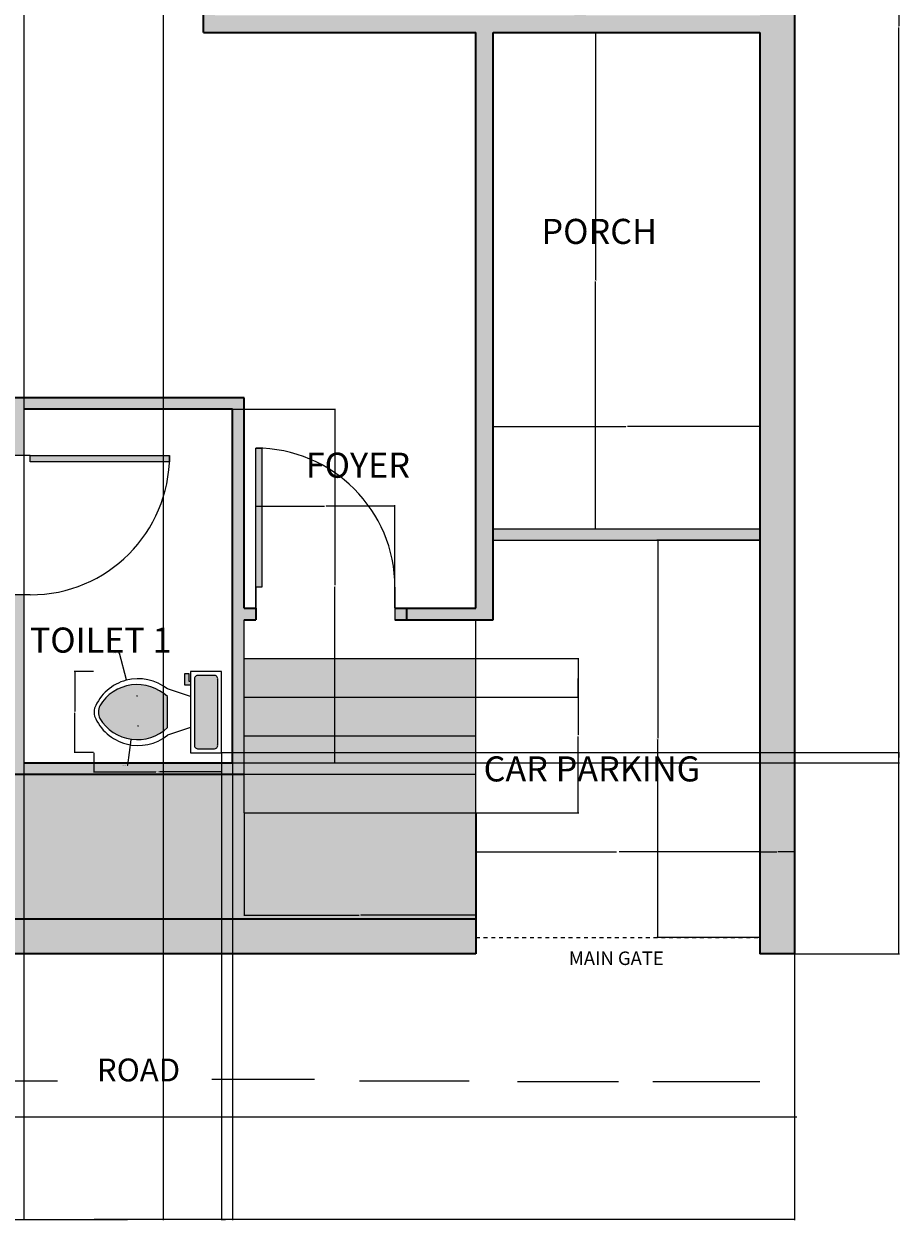
# Model space of a CAD drawing. Units: inches. Extents: x 1034 to 1730, y 674 to 1249.
# Tile 2 of 4: x 1503 to 1730, y 674 to 983. Entities that reach past the tile are written whole.
import ezdxf

# ---------------------------------------------------------------- set-up
doc = ezdxf.new("R2010")
doc.units = ezdxf.units.IN
doc.linetypes.add('JIS_02_1.0', pattern=[2, 1, -1])
for name, color, linetype, lineweight in [('A-ANNO-DIMS', 2, 'Continuous', 18), ('A-ANNO-TEXT', 7, 'Continuous', 18), ('A-AREA-IDEN', 7, 'Continuous', 18), ('A-DOOR', 4, 'Continuous', 25), ('A-FLOR', 7, 'Continuous', 25), ('A-FLOR-FIXT', 9, 'Continuous', 18), ('A-FLOR-FIXT-PATT', 7, 'Continuous', 13), ('A-FLOR-PATT', 8, 'Continuous', 13), ('A-FLOR-STRS', 7, 'Continuous', 25), ('A-FURN-PATT', 7, 'Continuous', 13), ('A-WALL', 7, 'Continuous', 35), ('A-WALL-PATT', 8, 'Continuous', 13), ('C-ROAD', 7, 'Continuous', 18), ('C-SITE-GATE', 4, 'JIS_02_1.0', 25)]:
    doc.layers.add(name, color=color, linetype=linetype, lineweight=lineweight)
for name, color, linetype, lineweight, true_color in [('A-DOOR-PATT', 17, 'Continuous', 13, 0x7b4636), ('A-FLOR-STRS-PATT', 253, 'Continuous', 13, 0xb3beaa), ('C-SITE-PATT', 18, 'Continuous', 13, 0x000000)]:
    doc.layers.add(name, color=color, linetype=linetype, lineweight=lineweight, true_color=true_color)
doc.styles.get("Standard").update_dxf_attribs({"font": 'arial.ttf'})
doc.dimstyles.get("Standard").update_dxf_attribs({"dimtxt": 0.18, "dimasz": 0.18, "dimexe": 0.18, "dimexo": 0.0625, "dimgap": 0.09, "dimtad": 0, "dimtih": 1, "dimtoh": 1, "dimdec": 4, "dimzin": 0, "dimdsep": 46, "dimtxsty": 'Standard', "dimcen": 0.09, "dimadec": 0, "dimazin": 0, "dimtfac": 1, "dimtdec": 4, "dimtofl": 0, "dimtmove": 0, "dimatfit": 3, "dimfxl": 1, "dimtolj": 1, "dimtzin": 0, "dimarcsym": 0})

# ---------------------------------------------------------------- blocks, each defined once
blk = doc.blocks.new('*U3')
for p, q in [((0, 0), (0, -6)), ((40, 0), (40, -6))]:
    blk.add_line(p, q)
blk.add_lwpolyline([(0, 0), (0, 40), (1.75, 40), (1.75, 0)], close=True)
blk.add_arc((0, 0), 40, 0, 90)
blk = doc.blocks.new('Toilet - top')
for p, q in [((9.5, -6), (9.5, -2)), ((-10, -8.5), (-8, -8.5)), ((-10, -9.5), (-10, -8.5)), ((-8, -8.5), (-8, -8)), ((-7, -8), (-7, -9.5)), ((-4, -8), (-6, -14)), ((4, -8), (6, -14)), ((-7, -9.5), (-10, -9.5)), ((4, -14), (-4, -14))]:
    blk.add_line(p, q)
blk.add_lwpolyline([(10.5, -8), (10.5, 0), (-10.5, 0), (-10.5, -8)], close=True)
for points in [[(-9.5, -2), (-9.5, -6)], [(8.5, -1), (-8.5, -1)], [(-8.5, -7), (8.5, -7)]]:
    blk.add_lwpolyline(points)
for centre, radius, start, end in [((-8.62, -1.88), 0.884, 81.8699, 188.1301), ((8.62, -1.88), 0.884, 351.8699, 98.1301), ((-8.62, -6.12), 0.884, 171.8699, 278.1301), ((8.62, -6.12), 0.884, 261.8699, 8.1301), ((3.52, -21.58), 12.17, 141.4691, 247.9714), ((4.2, -21.82), 11.33, 136.3677, 238.9468), ((-3.52, -21.58), 12.17, 292.0284, 38.5307), ((-4.2, -21.82), 11.33, 301.053, 43.6321), ((0, -27.88), 4, 245.7318, 294.2682), ((0, -29), 4, 254.8605, 285.1395)]:
    blk.add_arc(centre, radius, start, end)
blk = doc.blocks.new('*D10')
at = {"layer": 'A-ANNO-DIMS', "color": 0, "lineweight": -2, "transparency": 16777216}
for p, q in [((1521.14, 794.46), (1521.14, 789.39)), ((1554.18, 794.46), (1554.18, 789.39)), ((1521.32, 789.57), (1537.19, 789.57)), ((1554, 789.57), (1538.13, 789.57))]:
    blk.add_line(p, q, dxfattribs=at)
at = {"layer": 'A-ANNO-DIMS', "color": 0, "transparency": 16777216}
for points in [[(1521.32, 789.6), (1521.32, 789.54), (1521.14, 789.57)], [(1554, 789.6), (1554, 789.54), (1554.18, 789.57)]]:
    blk.add_solid(points, dxfattribs=at)
at = {"layer": 'Defpoints', "color": 0, "transparency": 16777216}
for p in [(1521.14, 794.53), (1554.18, 794.53), (1554.18, 789.57)]:
    blk.add_point(p, dxfattribs=at)
at = {"layer": 'A-ANNO-DIMS', "color": 0, "transparency": 16777216, "insert": (1537.66, 789.57), "char_height": 0.18, "attachment_point": 5}
blk.add_mtext('\\A1;WC 33', dxfattribs=at)
blk = doc.blocks.new('*D11')
at = {"layer": 'A-ANNO-DIMS', "color": 0, "lineweight": -2, "transparency": 16777216}
for p, q in [((1521.07, 815.53), (1516, 815.53)), ((1516.18, 815.35), (1516.18, 805.21)), ((1516.18, 794.71), (1516.18, 804.85)), ((1521.07, 794.53), (1516, 794.53))]:
    blk.add_line(p, q, dxfattribs=at)
at = {"layer": 'A-ANNO-DIMS', "color": 0, "transparency": 16777216}
for points in [[(1516.15, 815.35), (1516.21, 815.35), (1516.18, 815.53)], [(1516.15, 794.71), (1516.21, 794.71), (1516.18, 794.53)]]:
    blk.add_solid(points, dxfattribs=at)
at = {"layer": 'Defpoints', "color": 0, "transparency": 16777216}
for p in [(1521.14, 815.53), (1516.18, 794.53), (1521.14, 794.53)]:
    blk.add_point(p, dxfattribs=at)
at = {"layer": 'A-ANNO-DIMS', "color": 0, "transparency": 16777216, "insert": (1516.18, 805.03), "char_height": 0.18, "attachment_point": 5}
blk.add_mtext('\\A1;21', dxfattribs=at)
blk = doc.blocks.new('*D14')
at = {"layer": 'A-ANNO-DIMS', "color": 0, "lineweight": -2, "transparency": 16777216}
for p, q in [((1342.53, 742.36), (1342.53, 673.53)), ((1702.53, 742.36), (1702.53, 673.53)), ((1342.71, 673.71), (1522.24, 673.71)), ((1702.35, 673.71), (1522.82, 673.71))]:
    blk.add_line(p, q, dxfattribs=at)
at = {"layer": 'A-ANNO-DIMS', "color": 0, "transparency": 16777216}
for points in [[(1342.71, 673.74), (1342.71, 673.68), (1342.53, 673.71)], [(1702.35, 673.74), (1702.35, 673.68), (1702.53, 673.71)]]:
    blk.add_solid(points, dxfattribs=at)
at = {"layer": 'Defpoints', "color": 0, "transparency": 16777216}
for p in [(1342.53, 742.43), (1702.53, 742.43), (1702.53, 673.71)]:
    blk.add_point(p, dxfattribs=at)
at = {"layer": 'A-ANNO-DIMS', "color": 0, "transparency": 16777216, "insert": (1522.53, 673.71), "char_height": 0.18, "attachment_point": 5}
blk.add_mtext('\\A1;360', dxfattribs=at)
blk = doc.blocks.new('*D15')
at = {"layer": 'A-ANNO-DIMS', "color": 0, "lineweight": -2, "transparency": 16777216}
for p, q in [((1702.59, 1222.43), (1729.69, 1222.43)), ((1729.51, 1222.25), (1729.51, 982.61)), ((1729.51, 742.61), (1729.51, 982.24)), ((1702.59, 742.43), (1729.69, 742.43))]:
    blk.add_line(p, q, dxfattribs=at)
at = {"layer": 'A-ANNO-DIMS', "color": 0, "transparency": 16777216}
for points in [[(1729.48, 1222.25), (1729.54, 1222.25), (1729.51, 1222.43)], [(1729.48, 742.61), (1729.54, 742.61), (1729.51, 742.43)]]:
    blk.add_solid(points, dxfattribs=at)
at = {"layer": 'Defpoints', "color": 0, "transparency": 16777216}
for p in [(1702.53, 1222.43), (1729.51, 1222.43), (1702.53, 742.43)]:
    blk.add_point(p, dxfattribs=at)
at = {"layer": 'A-ANNO-DIMS', "color": 0, "transparency": 16777216, "insert": (1729.51, 982.43), "char_height": 0.18, "attachment_point": 5}
blk.add_mtext('\\A1;480', dxfattribs=at)
blk = doc.blocks.new('*D24')
at = {"layer": 'A-ANNO-DIMS', "color": 0, "lineweight": -2, "transparency": 16777216}
for p, q in [((1624.53, 852.56), (1624.53, 879.13)), ((1624.71, 878.95), (1658.81, 878.95)), ((1693.35, 878.95), (1659.25, 878.95)), ((1693.53, 852.56), (1693.53, 879.13))]:
    blk.add_line(p, q, dxfattribs=at)
at = {"layer": 'A-ANNO-DIMS', "color": 0, "transparency": 16777216}
for points in [[(1624.71, 878.98), (1624.71, 878.92), (1624.53, 878.95)], [(1693.35, 878.98), (1693.35, 878.92), (1693.53, 878.95)]]:
    blk.add_solid(points, dxfattribs=at)
at = {"layer": 'Defpoints', "color": 0, "transparency": 16777216}
for p in [(1693.53, 878.95), (1624.53, 852.5), (1693.53, 852.5)]:
    blk.add_point(p, dxfattribs=at)
at = {"layer": 'A-ANNO-DIMS', "color": 0, "transparency": 16777216, "insert": (1659.03, 878.95), "char_height": 0.18, "attachment_point": 5}
blk.add_mtext('\\A1;69', dxfattribs=at)
blk = doc.blocks.new('*D25')
at = {"layer": 'A-ANNO-DIMS', "color": 0, "lineweight": -2, "transparency": 16777216}
for p, q in [((1624.59, 980.93), (1651.16, 980.93)), ((1650.98, 980.75), (1650.98, 916.9)), ((1650.98, 852.68), (1650.98, 916.53)), ((1624.59, 852.5), (1651.16, 852.5))]:
    blk.add_line(p, q, dxfattribs=at)
at = {"layer": 'A-ANNO-DIMS', "color": 0, "transparency": 16777216}
for points in [[(1650.95, 980.75), (1651.01, 980.75), (1650.98, 980.93)], [(1650.95, 852.68), (1651.01, 852.68), (1650.98, 852.5)]]:
    blk.add_solid(points, dxfattribs=at)
at = {"layer": 'Defpoints', "color": 0, "transparency": 16777216}
for p in [(1624.53, 980.93), (1624.53, 852.5), (1650.98, 852.5)]:
    blk.add_point(p, dxfattribs=at)
at = {"layer": 'A-ANNO-DIMS', "color": 0, "transparency": 16777216, "insert": (1650.98, 916.71), "char_height": 0.18, "attachment_point": 5}
blk.add_mtext('\\A1;128.42', dxfattribs=at)
blk = doc.blocks.new('*D28')
at = {"layer": 'A-ANNO-DIMS', "color": 0, "lineweight": -2, "transparency": 16777216}
for p, q in [((1503.03, 1153.36), (1503.03, 673.53)), ((1539.03, 1153.36), (1539.03, 673.53)), ((1503.21, 673.71), (1520.81, 673.71)), ((1538.85, 673.71), (1521.25, 673.71))]:
    blk.add_line(p, q, dxfattribs=at)
at = {"layer": 'A-ANNO-DIMS', "color": 0, "transparency": 16777216}
for points in [[(1503.21, 673.74), (1503.21, 673.68), (1503.03, 673.71)], [(1538.85, 673.74), (1538.85, 673.68), (1539.03, 673.71)]]:
    blk.add_solid(points, dxfattribs=at)
at = {"layer": 'Defpoints', "color": 0, "transparency": 16777216}
for p in [(1503.03, 1153.43), (1539.03, 1153.43), (1539.03, 673.71)]:
    blk.add_point(p, dxfattribs=at)
at = {"layer": 'A-ANNO-DIMS', "color": 0, "transparency": 16777216, "insert": (1521.03, 673.71), "char_height": 0.18, "attachment_point": 5}
blk.add_mtext('\\A1;36', dxfattribs=at)
blk = doc.blocks.new('*D29')
at = {"layer": 'A-ANNO-DIMS', "color": 0, "lineweight": -2, "transparency": 16777216}
for p, q in [((1503.03, 791.86), (1503.03, 673.53)), ((1557.03, 791.86), (1557.03, 673.53)), ((1503.21, 673.71), (1529.81, 673.71)), ((1556.85, 673.71), (1530.25, 673.71))]:
    blk.add_line(p, q, dxfattribs=at)
at = {"layer": 'A-ANNO-DIMS', "color": 0, "transparency": 16777216}
for points in [[(1503.21, 673.74), (1503.21, 673.68), (1503.03, 673.71)], [(1556.85, 673.74), (1556.85, 673.68), (1557.03, 673.71)]]:
    blk.add_solid(points, dxfattribs=at)
at = {"layer": 'Defpoints', "color": 0, "transparency": 16777216}
for p in [(1503.03, 791.93), (1557.03, 791.93), (1557.03, 673.71)]:
    blk.add_point(p, dxfattribs=at)
at = {"layer": 'A-ANNO-DIMS', "color": 0, "transparency": 16777216, "insert": (1530.03, 673.71), "char_height": 0.18, "attachment_point": 5}
blk.add_mtext('\\A1;54', dxfattribs=at)
blk = doc.blocks.new('*D30')
at = {"layer": 'A-ANNO-DIMS', "color": 0, "lineweight": -2, "transparency": 16777216}
for p, q in [((1557.09, 883.43), (1583.66, 883.43)), ((1583.48, 883.25), (1583.48, 837.86)), ((1583.48, 792.11), (1583.48, 837.49)), ((1557.09, 791.93), (1583.66, 791.93))]:
    blk.add_line(p, q, dxfattribs=at)
at = {"layer": 'A-ANNO-DIMS', "color": 0, "transparency": 16777216}
for points in [[(1583.45, 883.25), (1583.51, 883.25), (1583.48, 883.43)], [(1583.45, 792.11), (1583.51, 792.11), (1583.48, 791.93)]]:
    blk.add_solid(points, dxfattribs=at)
at = {"layer": 'Defpoints', "color": 0, "transparency": 16777216}
for p in [(1557.03, 883.43), (1557.03, 791.93), (1583.48, 791.93)]:
    blk.add_point(p, dxfattribs=at)
at = {"layer": 'A-ANNO-DIMS', "color": 0, "transparency": 16777216, "insert": (1583.48, 837.68), "char_height": 0.18, "attachment_point": 5}
blk.add_mtext('\\A1;91.5', dxfattribs=at)
blk = doc.blocks.new('*D39')
at = {"layer": 'A-ANNO-DIMS', "color": 0, "lineweight": -2, "transparency": 16777216}
for p, q in [((1620.03, 742.49), (1620.03, 769.06)), ((1620.21, 768.88), (1656.46, 768.88)), ((1693.35, 768.88), (1657.1, 768.88)), ((1693.53, 742.49), (1693.53, 769.06))]:
    blk.add_line(p, q, dxfattribs=at)
at = {"layer": 'A-ANNO-DIMS', "color": 0, "transparency": 16777216}
for points in [[(1620.21, 768.91), (1620.21, 768.85), (1620.03, 768.88)], [(1693.35, 768.91), (1693.35, 768.85), (1693.53, 768.88)]]:
    blk.add_solid(points, dxfattribs=at)
at = {"layer": 'Defpoints', "color": 0, "transparency": 16777216}
for p in [(1693.53, 768.88), (1620.03, 742.43), (1693.53, 742.43)]:
    blk.add_point(p, dxfattribs=at)
at = {"layer": 'A-ANNO-DIMS', "color": 0, "transparency": 16777216, "insert": (1656.78, 768.88), "char_height": 0.18, "attachment_point": 5}
blk.add_mtext('\\A1;73.5', dxfattribs=at)
blk = doc.blocks.new('*D40')
at = {"layer": 'A-ANNO-DIMS', "color": 0, "lineweight": -2, "transparency": 16777216}
for p, q in [((1560.03, 778.86), (1560.03, 752.3)), ((1620.03, 778.86), (1620.03, 752.3)), ((1560.21, 752.48), (1589.81, 752.48)), ((1619.85, 752.48), (1590.25, 752.48))]:
    blk.add_line(p, q, dxfattribs=at)
at = {"layer": 'A-ANNO-DIMS', "color": 0, "transparency": 16777216}
for points in [[(1560.21, 752.51), (1560.21, 752.45), (1560.03, 752.48)], [(1619.85, 752.51), (1619.85, 752.45), (1620.03, 752.48)]]:
    blk.add_solid(points, dxfattribs=at)
at = {"layer": 'Defpoints', "color": 0, "transparency": 16777216}
for p in [(1560.03, 778.93), (1620.03, 778.93), (1560.03, 752.48)]:
    blk.add_point(p, dxfattribs=at)
at = {"layer": 'A-ANNO-DIMS', "color": 0, "transparency": 16777216, "insert": (1590.03, 752.48), "char_height": 0.18, "attachment_point": 5}
blk.add_mtext('\\A1;60', dxfattribs=at)
blk = doc.blocks.new('*D41')
at = {"layer": 'A-ANNO-DIMS', "color": 0, "lineweight": -2, "transparency": 16777216}
for p, q in [((1693.53, 742.49), (1693.53, 769.06)), ((1693.71, 768.88), (1697.88, 768.88)), ((1702.35, 768.88), (1698.18, 768.88)), ((1702.53, 742.49), (1702.53, 769.06))]:
    blk.add_line(p, q, dxfattribs=at)
at = {"layer": 'A-ANNO-DIMS', "color": 0, "transparency": 16777216}
for points in [[(1693.71, 768.91), (1693.71, 768.85), (1693.53, 768.88)], [(1702.35, 768.91), (1702.35, 768.85), (1702.53, 768.88)]]:
    blk.add_solid(points, dxfattribs=at)
at = {"layer": 'Defpoints', "color": 0, "transparency": 16777216}
for p in [(1702.53, 768.88), (1693.53, 742.43), (1702.53, 742.43)]:
    blk.add_point(p, dxfattribs=at)
at = {"layer": 'A-ANNO-DIMS', "color": 0, "transparency": 16777216, "insert": (1698.03, 768.88), "char_height": 0.18, "attachment_point": 5}
blk.add_mtext('\\A1;9', dxfattribs=at)
blk = doc.blocks.new('*D44')
at = {"layer": 'A-ANNO-DIMS', "color": 0, "lineweight": -2, "transparency": 16777216}
for p, q in [((1620.09, 818.93), (1646.66, 818.93)), ((1646.48, 818.75), (1646.48, 799.11)), ((1646.48, 779.11), (1646.48, 798.74)), ((1620.09, 778.93), (1646.66, 778.93))]:
    blk.add_line(p, q, dxfattribs=at)
at = {"layer": 'A-ANNO-DIMS', "color": 0, "transparency": 16777216}
for points in [[(1646.45, 818.75), (1646.51, 818.75), (1646.48, 818.93)], [(1646.45, 779.11), (1646.51, 779.11), (1646.48, 778.93)]]:
    blk.add_solid(points, dxfattribs=at)
at = {"layer": 'Defpoints', "color": 0, "transparency": 16777216}
for p in [(1620.03, 818.93), (1620.03, 778.93), (1646.48, 778.93)]:
    blk.add_point(p, dxfattribs=at)
at = {"layer": 'A-ANNO-DIMS', "color": 0, "transparency": 16777216, "insert": (1646.48, 798.93), "char_height": 0.18, "attachment_point": 5}
blk.add_mtext('\\A1;40', dxfattribs=at)
blk = doc.blocks.new('*D47')
at = {"layer": 'A-ANNO-DIMS', "color": 0, "lineweight": -2, "transparency": 16777216}
for p, q in [((1563.03, 831.99), (1563.03, 858.56)), ((1563.21, 858.38), (1580.81, 858.38)), ((1598.85, 858.38), (1581.25, 858.38)), ((1599.03, 831.99), (1599.03, 858.56))]:
    blk.add_line(p, q, dxfattribs=at)
at = {"layer": 'A-ANNO-DIMS', "color": 0, "transparency": 16777216}
for points in [[(1563.21, 858.41), (1563.21, 858.35), (1563.03, 858.38)], [(1598.85, 858.41), (1598.85, 858.35), (1599.03, 858.38)]]:
    blk.add_solid(points, dxfattribs=at)
at = {"layer": 'Defpoints', "color": 0, "transparency": 16777216}
for p in [(1599.03, 858.38), (1563.03, 831.93), (1599.03, 831.93)]:
    blk.add_point(p, dxfattribs=at)
at = {"layer": 'A-ANNO-DIMS', "color": 0, "transparency": 16777216, "insert": (1581.03, 858.38), "char_height": 0.18, "attachment_point": 5}
blk.add_mtext('\\A1;36', dxfattribs=at)
blk = doc.blocks.new('*D48')
at = {"layer": 'A-ANNO-DIMS', "color": 0, "lineweight": -2, "transparency": 16777216}
for p, q in [((1620.09, 818.93), (1646.66, 818.93)), ((1646.48, 818.75), (1646.48, 814.11)), ((1646.48, 809.11), (1646.48, 813.74)), ((1620.09, 808.93), (1646.66, 808.93))]:
    blk.add_line(p, q, dxfattribs=at)
at = {"layer": 'A-ANNO-DIMS', "color": 0, "transparency": 16777216}
for points in [[(1646.45, 818.75), (1646.51, 818.75), (1646.48, 818.93)], [(1646.45, 809.11), (1646.51, 809.11), (1646.48, 808.93)]]:
    blk.add_solid(points, dxfattribs=at)
at = {"layer": 'Defpoints', "color": 0, "transparency": 16777216}
for p in [(1620.03, 818.93), (1620.03, 808.93), (1646.48, 808.93)]:
    blk.add_point(p, dxfattribs=at)
at = {"layer": 'A-ANNO-DIMS', "color": 0, "transparency": 16777216, "insert": (1646.48, 813.93), "char_height": 0.18, "attachment_point": 5}
blk.add_mtext('\\A1;10', dxfattribs=at)
blk = doc.blocks.new('*D49')
at = {"layer": 'A-ANNO-DIMS', "color": 0, "lineweight": -2, "transparency": 16777216}
for p, q in [((1554.18, 794.46), (1554.18, 673.53)), ((1557.03, 791.86), (1557.03, 673.53)), ((1554.36, 673.71), (1555.21, 673.71)), ((1556.85, 673.71), (1556, 673.71))]:
    blk.add_line(p, q, dxfattribs=at)
at = {"layer": 'A-ANNO-DIMS', "color": 0, "transparency": 16777216}
for points in [[(1554.36, 673.74), (1554.36, 673.68), (1554.18, 673.71)], [(1556.85, 673.74), (1556.85, 673.68), (1557.03, 673.71)]]:
    blk.add_solid(points, dxfattribs=at)
at = {"layer": 'Defpoints', "color": 0, "transparency": 16777216}
for p in [(1554.18, 794.53), (1557.03, 791.93), (1557.03, 673.71)]:
    blk.add_point(p, dxfattribs=at)
at = {"layer": 'A-ANNO-DIMS', "color": 0, "transparency": 16777216, "insert": (1555.61, 673.71), "char_height": 0.18, "attachment_point": 5}
blk.add_mtext('\\A1;2.847', dxfattribs=at)
blk = doc.blocks.new('*D50')
at = {"layer": 'A-ANNO-DIMS', "color": 0, "lineweight": -2, "transparency": 16777216}
for p, q in [((1554.24, 794.53), (1729.69, 794.53)), ((1729.51, 794.35), (1729.51, 793.41)), ((1729.51, 792.11), (1729.51, 793.04)), ((1557.09, 791.93), (1729.69, 791.93))]:
    blk.add_line(p, q, dxfattribs=at)
at = {"layer": 'A-ANNO-DIMS', "color": 0, "transparency": 16777216}
for points in [[(1729.48, 794.35), (1729.54, 794.35), (1729.51, 794.53)], [(1729.48, 792.11), (1729.54, 792.11), (1729.51, 791.93)]]:
    blk.add_solid(points, dxfattribs=at)
at = {"layer": 'Defpoints', "color": 0, "transparency": 16777216}
for p in [(1554.18, 794.53), (1557.03, 791.93), (1729.51, 791.93)]:
    blk.add_point(p, dxfattribs=at)
at = {"layer": 'A-ANNO-DIMS', "color": 0, "transparency": 16777216, "insert": (1729.51, 793.23), "char_height": 0.18, "attachment_point": 5}
blk.add_mtext('\\A1;2.601', dxfattribs=at)
blk = doc.blocks.new('*D54')
at = {"layer": 'A-ANNO-DIMS', "color": 0, "lineweight": -2, "transparency": 16777216}
for p, q in [((1693.47, 849.5), (1666.9, 849.5)), ((1667.08, 849.32), (1667.08, 798.27)), ((1667.08, 746.86), (1667.08, 797.91)), ((1693.47, 746.68), (1666.9, 746.68))]:
    blk.add_line(p, q, dxfattribs=at)
at = {"layer": 'A-ANNO-DIMS', "color": 0, "transparency": 16777216}
for points in [[(1667.05, 849.32), (1667.11, 849.32), (1667.08, 849.5)], [(1667.05, 746.86), (1667.11, 746.86), (1667.08, 746.68)]]:
    blk.add_solid(points, dxfattribs=at)
at = {"layer": 'Defpoints', "color": 0, "transparency": 16777216}
for p in [(1667.08, 849.5), (1693.53, 849.5), (1693.53, 746.68)]:
    blk.add_point(p, dxfattribs=at)
at = {"layer": 'A-ANNO-DIMS', "color": 0, "transparency": 16777216, "insert": (1667.08, 798.09), "char_height": 0.18, "attachment_point": 5}
blk.add_mtext('\\A1;102.82', dxfattribs=at)
blk = doc.blocks.new('*D55')
at = {"layer": 'A-ANNO-DIMS', "color": 0, "lineweight": -2, "transparency": 16777216}
for p, q in [((1527.47, 820.34), (1527.65, 820.34)), ((1527.65, 820.34), (1529.46, 813.45)), ((1532.51, 801.51), (1532.69, 801.51)), ((1532.6, 801.42), (1532.6, 801.6))]:
    blk.add_line(p, q, dxfattribs=at)
at = {"layer": 'A-ANNO-DIMS', "color": 0, "transparency": 16777216}
blk.add_solid([(1529.49, 813.46), (1529.43, 813.44), (1529.51, 813.28)], dxfattribs=at)
at = {"layer": 'Defpoints', "color": 0, "transparency": 16777216}
for p in [(1529.51, 813.28), (1532.6, 801.51)]:
    blk.add_point(p, dxfattribs=at)
at = {"layer": 'A-ANNO-DIMS', "color": 0, "transparency": 16777216, "insert": (1526.8, 820.34), "char_height": 0.18, "attachment_point": 5}
blk.add_mtext('\\A1;2X R12.17', dxfattribs=at)
blk = doc.blocks.new('*D56')
at = {"layer": 'A-ANNO-DIMS', "color": 0, "lineweight": -2, "transparency": 16777216}
for p, q in [((1532.27, 809.23), (1532.45, 809.23)), ((1532.36, 809.14), (1532.36, 809.32)), ((1529.95, 791.26), (1530.83, 797.82)), ((1529.77, 791.26), (1529.95, 791.26))]:
    blk.add_line(p, q, dxfattribs=at)
at = {"layer": 'A-ANNO-DIMS', "color": 0, "transparency": 16777216}
blk.add_solid([(1530.8, 797.82), (1530.86, 797.82), (1530.85, 798)], dxfattribs=at)
at = {"layer": 'Defpoints', "color": 0, "transparency": 16777216}
for p in [(1532.36, 809.23), (1530.85, 798)]:
    blk.add_point(p, dxfattribs=at)
at = {"layer": 'A-ANNO-DIMS', "color": 0, "transparency": 16777216, "insert": (1529.09, 791.26), "char_height": 0.18, "attachment_point": 5}
blk.add_mtext('\\A1;2X R11.33', dxfattribs=at)

msp = doc.modelspace()

# ---------------------------------------------------------------- hatches: boundary and pattern name
at = {"layer": 'A-DOOR-PATT'}
h = msp.add_hatch(color=256, dxfattribs=at)
h.dxf.hatch_style = 1
h.paths.add_polyline_path([(1490.123, 922.4262), (1454.0839, 922.4262, 0.01094143), (1454.1184, 920.8495), (1490.123, 920.8495)])
h.paths.add_polyline_path([(1540.7238, 871.4262), (1504.6847, 871.4262), (1504.6847, 869.8495), (1540.6893, 869.8495, 0.01094143)])
h.paths.add_polyline_path([(1503.0288, 874.4262), (1495.5288, 874.4262), (1495.5288, 871.4262), (1503.0288, 871.4262)])
h.paths.add_polyline_path([(1503.0288, 835.3871), (1499.2788, 835.3871), (1495.5288, 835.4262), (1495.5288, 832.4262), (1503.0288, 832.4262)])
h.paths.add_polyline_path([(1564.6056, 873.3367, 0.01094143), (1563.0288, 873.3712), (1563.0288, 837.3321), (1564.6056, 837.3321)])
h.paths.add_polyline_path([(1602.0288, 831.9262), (1599.0288, 831.9262), (1599.0288, 828.9262), (1602.0288, 828.9262)])
h.paths.add_polyline_path([(1648.5288, 988.4262), (1645.5288, 988.4262), (1645.5288, 985.4262), (1648.5288, 985.4262)])
h.paths.add_polyline_path([(1689.9738, 989.9638), (1653.9347, 989.9638), (1653.9347, 988.3871), (1689.9738, 988.3871)])
h.paths.add_polyline_path([(1648.5288, 1027.4262), (1645.5288, 1027.4262), (1645.5288, 1024.4262), (1648.5288, 1024.4262)])
h.paths.add_polyline_path([(1590.9393, 1097.9638), (1554.9347, 1097.9638), (1554.9347, 1096.3871), (1590.9738, 1096.3871, 0.01094143)])
h.paths.add_polyline_path([(1549.5288, 1135.4262), (1545.0288, 1135.4262), (1545.0288, 1132.4262), (1549.5288, 1132.4262)])
h.paths.add_polyline_path([(1500.0288, 1135.4262), (1495.5288, 1135.4262), (1495.5288, 1132.4262), (1500.0288, 1132.4262)])
h.paths.add_polyline_path([(1490.123, 1098.0029), (1454.0839, 1098.0029), (1454.0839, 1096.4262), (1490.123, 1096.4262)])
h.paths.add_polyline_path([(1539.068, 1194.8712, 0.01094143), (1537.4912, 1194.8367), (1537.4912, 1158.8321), (1539.068, 1158.8321)])
at = {"layer": 'A-FLOR-FIXT-PATT'}
h = msp.add_hatch(color=256, dxfattribs=at)
h.dxf.hatch_style = 1
h.paths.add_polyline_path([(1522.659, 806.671, 0.21500378), (1522.659, 803.383, 0.4800795), (1540.182, 801.027), (1540.182, 809.027, 0.48007965)])
h.paths.add_polyline_path([(1553.182, 813.527, 0.50000012), (1552.182, 814.527), (1548.182, 814.527, 0.50000012), (1547.182, 813.527), (1547.182, 796.527, 0.50000012), (1548.182, 795.527), (1552.182, 795.527, 0.50000012), (1553.182, 796.527)])
h.paths.add_polyline_path([(1545.682, 815.027), (1544.682, 815.027), (1544.682, 812.027), (1546.182, 812.027), (1546.182, 813.027), (1545.682, 813.027)])
at = {"layer": 'A-FLOR-PATT'}
h = msp.add_hatch(color=256, dxfattribs=at)
h.dxf.hatch_style = 1
h.paths.add_polyline_path([(1693.5288, 852.5025), (1624.5288, 852.5025), (1624.5288, 849.5025), (1693.5288, 849.5025)])
at = {"layer": 'A-FLOR-STRS-PATT'}
h = msp.add_hatch(color=256, dxfattribs=at)
h.dxf.hatch_style = 1
h.paths.add_polyline_path([(1620.0288, 818.9262), (1560.0288, 818.9262), (1560.0288, 808.9262), (1620.0288, 808.9262)])
h.paths.add_polyline_path([(1620.0288, 808.9262), (1560.0288, 808.9262), (1560.0288, 798.9262), (1620.0288, 798.9262)])
h.paths.add_polyline_path([(1620.0288, 798.9262), (1560.0288, 798.9262), (1560.0288, 788.9262), (1620.0288, 788.9262)])
h.paths.add_polyline_path([(1620.0288, 788.9262), (1560.0288, 788.9262), (1560.0288, 778.9262), (1620.0288, 778.9262)])
at = {"layer": 'A-FURN-PATT'}
h = msp.add_hatch(color=256, dxfattribs=at)
h.dxf.hatch_style = 1
h.paths.add_polyline_path([(1414.278, 838.2731), (1381.0078, 838.2731), (1381.0078, 828.2392), (1372.5582, 828.2392), (1372.5582, 798.6657), (1414.278, 798.6657)])
h.paths.add_polyline_path([(1370.9739, 828.2392), (1372.2941, 829.5594), (1372.2941, 832.9921), (1362.2603, 832.9921), (1362.2603, 819.2615), (1370.9739, 819.2615)], flags=17)
h.paths.add_polyline_path([(1370.9739, 817.6772), (1362.2603, 817.6772), (1362.2603, 803.9467), (1370.9739, 803.9467)], flags=17)
h.paths.add_polyline_path([(1367.0568, 1198.6055), (1368.377, 1199.9257), (1368.377, 1203.3584), (1358.3431, 1203.3584), (1358.3431, 1189.6278), (1367.0568, 1189.6278)], flags=17)
h.paths.add_polyline_path([(1367.0568, 1188.0435), (1358.3431, 1188.0435), (1358.3431, 1174.3129), (1367.0568, 1174.3129)], flags=17)
h.paths.add_polyline_path([(1410.3609, 1208.6394), (1377.0906, 1208.6394), (1377.0906, 1198.6055), (1368.6411, 1198.6055), (1368.6411, 1169.032), (1410.3609, 1169.032)])
h.paths.add_polyline_path([(1678.2824, 1203.4604), (1636.5626, 1203.4604), (1636.5626, 1163.853), (1669.8329, 1163.853), (1669.8329, 1173.8868), (1678.2824, 1173.8868)])
h.paths.add_polyline_path([(1688.5804, 1182.8645), (1679.8667, 1182.8645), (1679.8667, 1173.8868), (1678.5465, 1172.5666), (1678.5465, 1169.1339), (1688.5804, 1169.1339)], flags=17)
h.paths.add_polyline_path([(1367.0568, 1174.3129), (1358.3431, 1174.3129), (1358.3431, 1188.0435), (1367.0568, 1188.0435), (1367.0568, 1189.6278), (1358.3431, 1189.6278), (1358.3431, 1203.3584), (1368.377, 1203.3584), (1368.377, 1199.9257), (1377.0906, 1208.6394), (1357.551, 1208.6394), (1357.551, 1169.032), (1367.0568, 1169.032)])
h.paths.add_polyline_path([(1688.5804, 1198.1794), (1679.8667, 1198.1794), (1679.8667, 1184.4488), (1688.5804, 1184.4488)], flags=17)
h.paths.add_polyline_path([(1689.3725, 1203.4604), (1679.8667, 1203.4604), (1679.8667, 1198.1794), (1688.5804, 1198.1794), (1688.5804, 1184.4488), (1679.8667, 1184.4488), (1679.8667, 1182.8645), (1688.5804, 1182.8645), (1688.5804, 1169.1339), (1678.5465, 1169.1339), (1678.5465, 1172.5666), (1669.8329, 1163.853), (1689.3725, 1163.853)])
h.paths.add_polyline_path([(1370.9739, 803.9467), (1362.2603, 803.9467), (1362.2603, 817.6772), (1370.9739, 817.6772), (1370.9739, 819.2615), (1362.2603, 819.2615), (1362.2603, 832.9921), (1372.2941, 832.9921), (1372.2941, 829.5594), (1381.0078, 838.2731), (1361.4681, 838.2731), (1361.4681, 798.6657), (1370.9739, 798.6657)])
h.paths.add_polyline_path([(1586.4252, 1162.5974), (1646.7165, 1162.5974), (1646.7165, 1172.6784), (1586.4252, 1172.6784)], flags=9)
h.paths.add_polyline_path([(1574.2942, 863.9077), (1611.4062, 863.9077), (1611.4062, 873.9821), (1574.2942, 873.9821)], flags=9)
h.paths.add_polyline_path([(1502.8652, 818.6383), (1550.5629, 818.6383), (1550.5629, 828.7127), (1502.8652, 828.7127)], flags=9)
h.paths.add_polyline_path([(1367.7365, 861.2327), (1425.5064, 861.2327), (1425.5064, 871.3071), (1367.7365, 871.3071)], flags=9)
h.paths.add_polyline_path([(1409.7909, 1010.2859), (1487.2071, 1010.2859), (1487.2071, 1020.3537), (1409.7909, 1020.3537)], flags=9)
h.paths.add_polyline_path([(1499.9637, 1199.6865), (1545.1423, 1199.6865), (1545.1423, 1209.7608), (1499.9637, 1209.7608)], flags=9)
h.paths.add_polyline_path([(1378.5639, 1158.2313), (1436.3338, 1158.2313), (1436.3338, 1168.3057), (1378.5639, 1168.3057)], flags=9)
at = {"layer": 'A-WALL-PATT'}
h = msp.add_hatch(color=256, dxfattribs=at)
h.dxf.hatch_style = 1
h.paths.add_polyline_path([(1351.5288, 1213.4262), (1495.5288, 1213.4262), (1495.5288, 1135.4262), (1500.0288, 1135.4262), (1500.0288, 1148.9262), (1503.0288, 1148.9262), (1503.0288, 1153.4262), (1500.0288, 1153.4262), (1500.0288, 1213.4262), (1545.0288, 1213.4262), (1545.0288, 1153.4262), (1539.0288, 1153.4262), (1539.0288, 1148.9262), (1545.0288, 1148.9262), (1545.0288, 1135.4262), (1549.5288, 1135.4262), (1549.5288, 1213.4262), (1693.5288, 1213.4262), (1693.5288, 1093.4262), (1549.5288, 1093.4262), (1549.5288, 1096.4262), (1545.0288, 1096.4262), (1545.0288, 1088.9262), (1549.5288, 1088.9262), (1549.5288, 1064.9262), (1552.5288, 1064.9262), (1552.5288, 1088.9262), (1645.5288, 1088.9262), (1645.5288, 1027.4262), (1648.5288, 1027.4262), (1648.5288, 1088.9262), (1693.5288, 1088.9262), (1693.5288, 985.4262), (1552.5288, 985.4262), (1552.5288, 1004.9262), (1549.5288, 1004.9262), (1549.5288, 980.9262), (1620.0288, 980.9262), (1620.0288, 831.9262), (1602.0288, 831.9262), (1602.0288, 828.9262), (1624.5288, 828.9262), (1624.5288, 980.9262), (1693.5288, 980.9262), (1693.5288, 742.4262), (1702.5288, 742.4262), (1702.5288, 1222.4262), (1342.5288, 1222.4262), (1342.5288, 742.4262), (1620.0288, 742.4262), (1620.0288, 751.4262), (1351.5288, 751.4262), (1351.5288, 788.9262), (1560.0288, 788.9262), (1560.0288, 828.9262), (1563.0288, 828.9262), (1563.0288, 831.9262), (1560.0288, 831.9262), (1560.0288, 886.4262), (1500.0288, 886.4262), (1495.5288, 886.4262), (1495.5288, 874.4262), (1503.0288, 874.4262), (1503.0288, 883.4262), (1557.0288, 883.4262), (1557.0288, 791.9262), (1503.0288, 791.9262), (1503.0288, 832.4262), (1495.5288, 832.4262), (1495.5288, 793.4262), (1351.5288, 793.4262), (1351.5288, 925.4262), (1495.5288, 925.4262), (1495.5288, 922.4262), (1500.0288, 922.4262), (1500.0288, 929.9262), (1351.5288, 929.9262), (1351.5288, 1088.9262), (1500.0288, 1088.9262), (1500.0288, 1096.4262), (1495.5288, 1096.4262), (1495.5288, 1093.4262), (1351.5288, 1093.4262)])
at = {"layer": 'C-SITE-PATT'}
h = msp.add_hatch(color=256, dxfattribs=at)
h.dxf.hatch_style = 1
h.paths.add_polyline_path([(1620.0288, 778.9262), (1560.0288, 778.9262), (1560.0288, 788.9262), (1351.5288, 788.9262), (1351.5288, 751.4262), (1620.0288, 751.4262)])

# ---------------------------------------------------------------- linework, layer by layer
at = {"layer": 'A-DOOR'}
msp.add_line((1599.0288, 831.9262), (1599.0288, 828.9262), dxfattribs=at)
at = {"layer": 'A-FLOR'}
for p, q in [((1624.5288, 852.5025), (1693.5288, 852.5025)), ((1624.5288, 849.5025), (1693.5288, 849.5025))]:
    msp.add_line(p, q, dxfattribs=at)
at = {"layer": 'A-FLOR-STRS'}
for p, q in [((1560.0288, 778.9262), (1560.0288, 828.9262)), ((1620.0288, 778.9262), (1620.0288, 828.9262)), ((1560.0288, 818.9262), (1620.0288, 818.9262)), ((1560.0288, 808.9262), (1620.0288, 808.9262)), ((1560.0288, 798.9262), (1620.0288, 798.9262)), ((1560.0288, 788.9262), (1620.0288, 788.9262)), ((1560.0288, 778.9262), (1620.0288, 778.9262))]:
    msp.add_line(p, q, dxfattribs=at)
at = {"layer": 'A-WALL'}
for p, q in [((1549.5288, 980.9262), (1549.5288, 1004.9262)), ((1549.5288, 980.9262), (1620.0288, 980.9262)), ((1620.0288, 831.9262), (1620.0288, 980.9262)), ((1624.5288, 828.9262), (1624.5288, 980.9262)), ((1624.5288, 980.9262), (1693.5288, 980.9262)), ((1693.5288, 980.9262), (1693.5288, 742.4262)), ((1560.0288, 886.4262), (1500.0288, 886.4262)), ((1560.0288, 831.9262), (1560.0288, 886.4262)), ((1557.0288, 883.4262), (1503.0288, 883.4262)), ((1557.0288, 791.9262), (1557.0288, 883.4262)), ((1560.0288, 831.9262), (1563.0288, 831.9262)), ((1563.0288, 831.9262), (1563.0288, 828.9262)), ((1599.0288, 831.9262), (1620.0288, 831.9262)), ((1602.0288, 831.9262), (1602.0288, 828.9262)), ((1560.0288, 828.9262), (1563.0288, 828.9262)), ((1599.0288, 828.9262), (1624.5288, 828.9262)), ((1503.0288, 791.9262), (1557.0288, 791.9262)), ((1351.5288, 788.9262), (1560.0288, 788.9262)), ((1620.0288, 778.9262), (1620.0288, 742.4262)), ((1620.0288, 751.4262), (1351.5288, 751.4262))]:
    msp.add_line(p, q, dxfattribs=at)
msp.add_lwpolyline([(1620.0288, 742.4262), (1342.5288, 742.4262), (1342.5288, 1222.4262), (1702.5288, 1222.4262), (1702.5288, 742.4262), (1693.5288, 742.4262)], dxfattribs=at)
at = {"layer": 'C-ROAD'}
for p, q in [((1494.9352, 709.5884), (1511.7588, 709.5884)), ((1551.6474, 710.0102), (1578.2669, 710.0102)), ((1589.8998, 709.5913), (1618.2408, 709.5913)), ((1630.8161, 709.3783), (1656.9727, 709.3783)), ((1665.8593, 709.3783), (1693.5249, 709.3783)), ((1703.0641, 700.1632), (1350.0973, 700.1632))]:
    msp.add_line(p, q, dxfattribs=at)
at = {"layer": 'C-SITE-GATE'}
msp.add_line((1620.0288, 746.6779), (1693.5288, 746.6779), dxfattribs=at)

# ---------------------------------------------------------------- block references
at = {"layer": 'A-DOOR', "xscale": 0.9009776753840846, "yscale": 0.9009776753840846, "zscale": 0.9009776753840846}
msp.add_blockref('*U3', (1563.0288, 837.3321), dxfattribs=at)
at = {"layer": 'A-DOOR', "xscale": 0.9009776753840846, "yscale": 0.9009776753840846, "zscale": 0.9009776753840846, "rotation": 270}
msp.add_blockref('*U3', (1504.6847, 871.4262), dxfattribs=at)
at = {"layer": 'A-FLOR-FIXT', "rotation": 270}
msp.add_blockref('Toilet - top', (1554.182, 805.027), dxfattribs=at)

# ---------------------------------------------------------------- texts
at = {"layer": 'A-ANNO-TEXT'}
for s, height, p in [('MAIN GATE', 3.49928, (1644.0884, 739.5602)), ('ROAD ', 5.90785, (1521.9198, 709.4352))]:
    msp.add_text(s, height=height, dxfattribs=at).set_placement(p)
at = {"layer": 'A-AREA-IDEN'}
for s, height, p in [('PORCH ', 6.49045, (1636.9973, 926.2231)), ('FOYER ', 6.49045, (1575.9732, 865.6974)), ('TOILET 1  ', 6.49045, (1504.5442, 820.4281)), ('CAR PARKING ', 6.490455, (1622.0163, 787.0824))]:
    msp.add_text(s, height=height, dxfattribs=at).set_placement(p)

# ---------------------------------------------------------------- dimensions: what is measured, and where the dimension line sits
at = {"layer": 'A-ANNO-DIMS'}
for base, p1, p2, angle, override, picture, middle in [((1729.5141, 1222.4262), (1702.5288, 742.4262), (1702.5288, 1222.4262), 90, {"dimdec": 0, "dimlfac": 1, "dimrnd": 0, "dimzin": 0, "dimdsep": 46, "dimlunit": 2}, '*D15', (1729.5141, 982.4262)), ((1650.9788, 852.5025), (1624.5288, 980.9262), (1624.5288, 852.5025), 270, {"dimdec": 2, "dimlfac": 1, "dimrnd": 0, "dimzin": 0, "dimdsep": 46, "dimlunit": 2}, '*D25', (1650.9788, 916.7143)), ((1583.4788, 791.9262), (1557.0288, 883.4262), (1557.0288, 791.9262), 270, {"dimdec": 1, "dimlfac": 1, "dimrnd": 0, "dimzin": 0, "dimdsep": 46, "dimlunit": 2}, '*D30', (1583.4788, 837.6762)), ((1693.5288, 878.9525), (1624.5288, 852.5025), (1693.5288, 852.5025), 0, {"dimdec": 0, "dimlfac": 1, "dimrnd": 0, "dimzin": 0, "dimdsep": 46, "dimlunit": 2}, '*D24', (1659.0288, 878.9525)), ((1667.0788, 849.5025), (1693.5288, 746.6779), (1693.5288, 849.5025), 90, {"dimdec": 2, "dimlfac": 1, "dimrnd": 0, "dimzin": 0, "dimdsep": 46, "dimlunit": 2}, '*D54', (1667.0788, 798.0902)), ((1646.4788, 778.9262), (1620.0288, 818.9262), (1620.0288, 778.9262), 270, {"dimdec": 0, "dimlfac": 1, "dimrnd": 0, "dimzin": 0, "dimdsep": 46, "dimlunit": 2}, '*D44', (1646.4788, 798.9262)), ((1646.4788, 808.9262), (1620.0288, 818.9262), (1620.0288, 808.9262), 270, {"dimdec": 0, "dimlfac": 1, "dimrnd": 0, "dimzin": 0, "dimdsep": 46, "dimlunit": 2}, '*D48', (1646.4788, 813.9262)), ((1516.1788, 794.527), (1521.1358, 815.527), (1521.1358, 794.527), 270, {"dimdec": 0, "dimlfac": 1, "dimrnd": 0, "dimzin": 0, "dimdsep": 46, "dimlunit": 2}, '*D11', (1516.1788, 805.027)), ((1729.5141, 791.9262), (1554.182, 794.527), (1557.0288, 791.9262), 90, {"dimdec": 3, "dimlfac": 1, "dimrnd": 0, "dimzin": 0, "dimdsep": 46, "dimlunit": 2}, '*D50', (1729.5141, 793.2266)), ((1560.0288, 752.4762), (1620.0288, 778.9262), (1560.0288, 778.9262), 180, {"dimdec": 0, "dimlfac": 1, "dimrnd": 0, "dimzin": 0, "dimdsep": 46, "dimlunit": 2}, '*D40', (1590.0288, 752.4762))]:
    dim = msp.add_linear_dim(base=base, p1=p1, p2=p2, angle=angle, dimstyle='Standard', override=override, dxfattribs=at)
    dim.commit()
    dim.dimension.update_dxf_attribs({"geometry": picture, "text_midpoint": middle})
for base, p1, p2, override, picture, middle in [((1539.0288, 673.7132), (1503.0288, 1153.4262), (1539.0288, 1153.4262), {"dimdec": 0, "dimlfac": 1, "dimrnd": 0, "dimzin": 0, "dimdsep": 46, "dimlunit": 2}, '*D28', (1521.0288, 673.7132)), ((1599.0288, 858.3762), (1563.0288, 831.9262), (1599.0288, 831.9262), {"dimdec": 0, "dimlfac": 1, "dimrnd": 0, "dimzin": 0, "dimdsep": 46, "dimlunit": 2}, '*D47', (1581.0288, 858.3762)), ((1557.0288, 673.7132), (1554.182, 794.527), (1557.0288, 791.9262), {"dimdec": 3, "dimlfac": 1, "dimrnd": 0, "dimzin": 0, "dimdsep": 46, "dimlunit": 2}, '*D49', (1555.6054, 673.7132)), ((1557.0288, 673.7132), (1503.0288, 791.9262), (1557.0288, 791.9262), {"dimdec": 0, "dimlfac": 1, "dimrnd": 0, "dimzin": 0, "dimdsep": 46, "dimlunit": 2}, '*D29', (1530.0288, 673.7132)), ((1693.5288, 768.8762), (1620.0288, 742.4262), (1693.5288, 742.4262), {"dimdec": 1, "dimlfac": 1, "dimrnd": 0, "dimzin": 0, "dimdsep": 46, "dimlunit": 2}, '*D39', (1656.7788, 768.8762)), ((1702.5288, 768.8762), (1693.5288, 742.4262), (1702.5288, 742.4262), {"dimdec": 0, "dimlfac": 1, "dimrnd": 0, "dimzin": 0, "dimdsep": 46, "dimlunit": 2}, '*D41', (1698.0288, 768.8762)), ((1702.5288, 673.7132), (1342.5288, 742.4262), (1702.5288, 742.4262), {"dimdec": 0, "dimlfac": 1, "dimrnd": 0, "dimzin": 0, "dimdsep": 46, "dimlunit": 2}, '*D14', (1522.5288, 673.7132))]:
    dim = msp.add_linear_dim(base=base, p1=p1, p2=p2, dimstyle='Standard', override=override, dxfattribs=at)
    dim.commit()
    dim.dimension.update_dxf_attribs({"geometry": picture, "text_midpoint": middle})
for center, mpoint, picture, middle in [((1532.6015, 801.5075), (1529.509, 813.277), '*D55', (1526.7987, 820.3387)), ((1532.3646, 809.2269), (1530.855, 797.9988), '*D56', (1529.0944, 791.2619))]:
    dim = msp.add_radius_dim(center=center, mpoint=mpoint, text='2X <>', dimstyle='Standard', override={"dimdec": 2, "dimlfac": 1, "dimrnd": 0, "dimzin": 0, "dimdsep": 46, "dimlunit": 2}, dxfattribs=at)
    dim.commit()
    dim.dimension.update_dxf_attribs({"geometry": picture, "text_midpoint": middle, "dimtype": 164})
dim = msp.add_linear_dim(base=(1554.182, 789.5701), p1=(1521.1358, 794.527), p2=(1554.182, 794.527), text='WC <>', dimstyle='Standard', override={"dimdec": 0, "dimlfac": 1, "dimrnd": 0, "dimzin": 0, "dimdsep": 46, "dimlunit": 2}, dxfattribs=at)
dim.commit()
dim.dimension.update_dxf_attribs({"geometry": '*D10', "text_midpoint": (1537.6589, 789.5701)})

doc.saveas('drawing.dxf')
